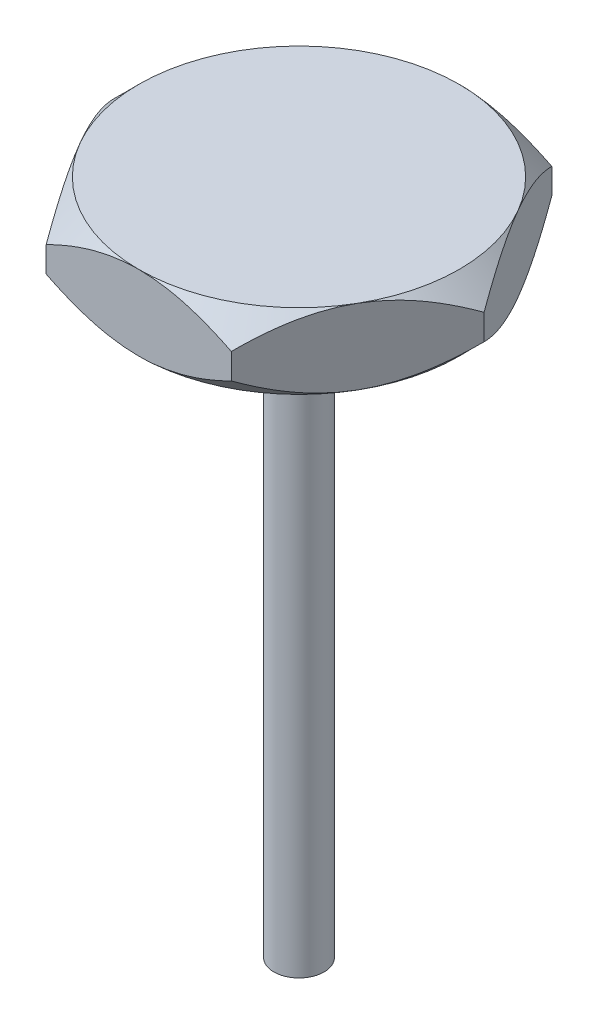
from build123d import *

# Parameters (mm, degrees)
HEX_HEAD_DEPTH                   = 3.75
HEAD_CHAMFER_A_PROFILE_OUTSIDE_W = 32.922
HEAD_CHAMFER_A_PROFILE_OUTSIDE_H = 30.446
HEAD_CHAMFER_A_PROFILE_OUTSIDE_R = 8
HEAD_CHAMFER_A_45DEG_DEPTH       = 3.75
HEAD_CHAMFER_A_45DEG_DRAFT       = -45
HEAD_CHAMFER_B_PROFILE_OUTSIDE_W = 32.922
HEAD_CHAMFER_B_PROFILE_OUTSIDE_H = 30.446
HEAD_CHAMFER_B_PROFILE_OUTSIDE_R = 8
HEAD_CHAMFER_B_45DEG_DEPTH       = 3.75
HEAD_CHAMFER_B_45DEG_DRAFT       = -45
SHANK_PROFILE_2_5_R              = 1.25
SHANK_2_5X30_DEPTH               = 30


with BuildPart() as part:
    # Hex Head Profile → Hex Head (new body)
    with BuildSketch(Plane(origin=(0, 0, 0), x_dir=(1, 0, 0), z_dir=(0, 1, 0))):
        Polygon((4.618802154, -8), (9.237604307, 0), (4.618802154, 8), (-4.618802154, 8), (-9.237604307, 0), (-4.618802154, -8), align=None)
    extrude(amount=HEX_HEAD_DEPTH)


with BuildPart() as head_chamfer_a_45deg_tool:
    # Head Chamfer A Profile outside → Head Chamfer A 45deg (with draft: the straight prism first)
    with BuildSketch(Plane(origin=(0, 3.75, 0), x_dir=(1, 0, 0), z_dir=(0, 1, 0))):
        Rectangle(HEAD_CHAMFER_A_PROFILE_OUTSIDE_W, HEAD_CHAMFER_A_PROFILE_OUTSIDE_H)
        Circle(HEAD_CHAMFER_A_PROFILE_OUTSIDE_R, mode=Mode.SUBTRACT)
    extrude(amount=-HEAD_CHAMFER_A_45DEG_DEPTH)
    # Head Chamfer A 45deg: the draft: its side faces are tilted about the plane it starts from
    head_chamfer_a_45deg_sides = [head_chamfer_a_45deg_tool.faces().sort_by_distance(p)[0] for p in [
        (0, 1.875, 15.223),
        (16.461, 1.875, 0),
        (0, 1.875, -15.223),
        (-16.461, 1.875, 0),
        (-8, 1.875, 0),
    ]]
    draft(head_chamfer_a_45deg_sides, Plane(origin=(0, 3.75, 0), x_dir=(1, 0, 0), z_dir=(0, 1, 0)), HEAD_CHAMFER_A_45DEG_DRAFT)


with BuildPart() as part_1:
    add(part.part)

    # Head Chamfer A 45deg: cut by head_chamfer_a_45deg_tool
    add(head_chamfer_a_45deg_tool.part, mode=Mode.SUBTRACT)


with BuildPart() as head_chamfer_b_45deg_tool:
    # Head Chamfer B Profile outside → Head Chamfer B 45deg (with draft: the straight prism first)
    with BuildSketch(Plane.XZ):
        Rectangle(HEAD_CHAMFER_B_PROFILE_OUTSIDE_W, HEAD_CHAMFER_B_PROFILE_OUTSIDE_H)
        Circle(HEAD_CHAMFER_B_PROFILE_OUTSIDE_R, mode=Mode.SUBTRACT)
    extrude(amount=-HEAD_CHAMFER_B_45DEG_DEPTH)
    # Head Chamfer B 45deg: the draft: its side faces are tilted about the plane it starts from
    head_chamfer_b_45deg_sides = [head_chamfer_b_45deg_tool.faces().sort_by_distance(p)[0] for p in [
        (0, 1.875, -15.223),
        (16.461, 1.875, 0),
        (0, 1.875, 15.223),
        (-16.461, 1.875, 0),
        (-8, 1.875, 0),
    ]]
    draft(head_chamfer_b_45deg_sides, Plane.XZ, HEAD_CHAMFER_B_45DEG_DRAFT)


with BuildPart() as part_2:
    add(part_1.part)

    # Head Chamfer B 45deg: cut by head_chamfer_b_45deg_tool
    add(head_chamfer_b_45deg_tool.part, mode=Mode.SUBTRACT)

    # Shank Profile Ø2.5 → Shank Ø2.5x30 (add)
    with BuildSketch(Plane.XZ):
        with Locations(Location((0, 0, 0), (0, 0, 90))):
            Circle(SHANK_PROFILE_2_5_R)
    extrude(amount=SHANK_2_5X30_DEPTH)


solid = part_2.part
